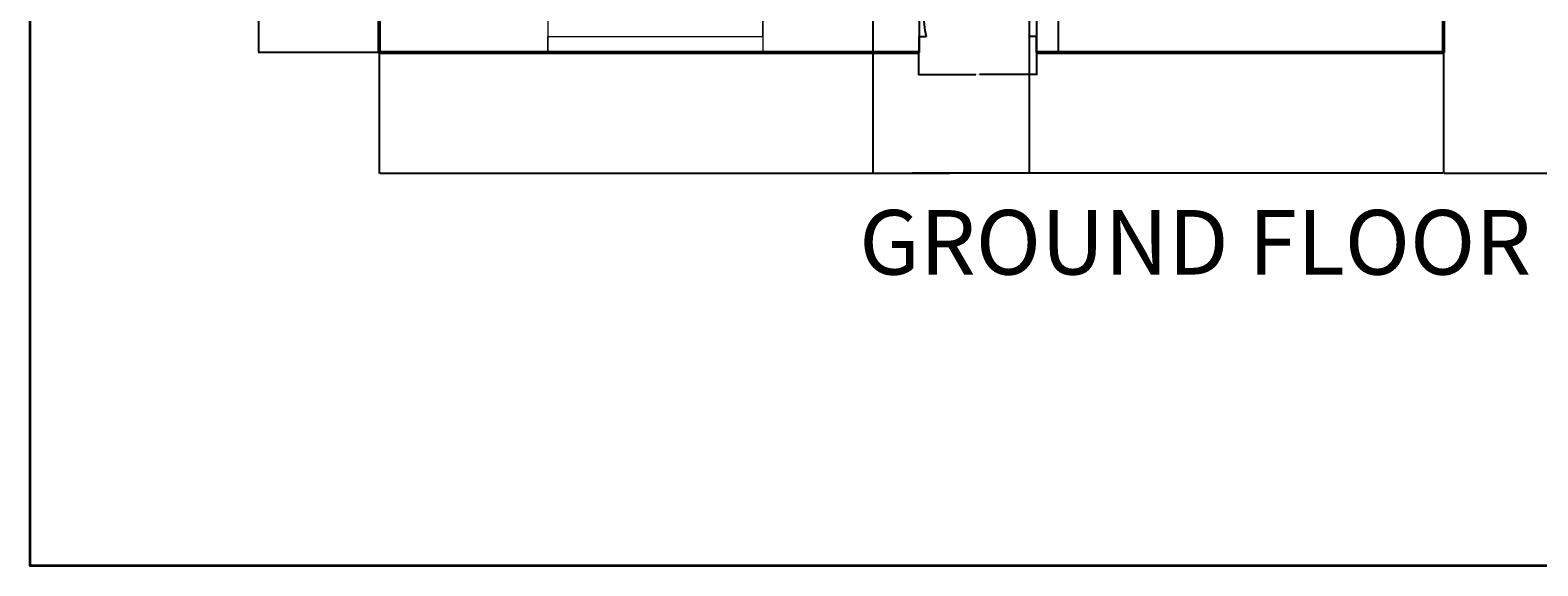
# Model space of a CAD drawing. Units: inches. Extents: x 2215 to 3724, y 1009 to 2124.
# Tile 1 of 11: x 2215 to 2636, y 1009 to 1158. Entities that reach past the tile are written whole.
import ezdxf

# ---------------------------------------------------------------- set-up
doc = ezdxf.new("R2010")
doc.units = ezdxf.units.IN
for name, color, linetype, lineweight in [('A-ANNO-DIMS', 2, 'Continuous', 18), ('A-ANNO-TEXT', 7, 'Continuous', 25), ('A-ANNO-TTLB', 7, 'Continuous', 35), ('A-DOOR', 3, 'Continuous', 25), ('A-GLAZ', 4, 'Continuous', 18), ('A-WALL', 7, 'Continuous', 50)]:
    doc.layers.add(name, color=color, linetype=linetype, lineweight=lineweight)
doc.styles.get("Standard").update_dxf_attribs({"font": 'arial.ttf'})
doc.dimstyles.get("Standard").update_dxf_attribs({"dimtxt": 0.18, "dimasz": 0.18, "dimexe": 0.18, "dimexo": 0.0625, "dimgap": 0.09, "dimtad": 0, "dimtih": 1, "dimtoh": 1, "dimdec": 4, "dimzin": 0, "dimdsep": 46, "dimtxsty": 'Standard', "dimcen": 0.09, "dimadec": 0, "dimazin": 0, "dimtfac": 1, "dimtdec": 4, "dimtofl": 0, "dimtmove": 0, "dimatfit": 3, "dimfxl": 1, "dimtolj": 1, "dimtzin": 0, "dimarcsym": 0})

# ---------------------------------------------------------------- blocks, each defined once
blk = doc.blocks.new('DOOR-FRONT-SINGLE')
for p, q in [((30.79, 4.5), (30.79, 40.5)), ((0, 9), (0, 0)), ((32.79, 9), (32.79, 0)), ((0, 0), (0, 4.5)), ((0, 4.5), (2, 4.5)), ((32.79, 4.5), (30.79, 4.5)), ((32.79, 0), (32.79, 4.5))]:
    blk.add_line(p, q)
blk.add_arc((30.39, 11.3), 29.2, 89.2162, 193.4744)
blk = doc.blocks.new('WIN-60-FRONT')
for p, q in [((0, 9), (0, 9)), ((0, 9), (0, 0)), ((60, 4.5), (60, 9)), ((60, 9), (60, 0)), ((0, 0), (0, 4.5)), ((0, 4.5), (60, 4.5))]:
    blk.add_line(p, q)
blk = doc.blocks.new('*D67')
at = {"layer": 'A-ANNO-DIMS', "color": 0, "lineweight": -2, "transparency": 16777216}
for p, q in [((2496.34, 1192.62), (2502.55, 1192.62)), ((2502.37, 1192.44), (2502.37, 1172.49)), ((2502.37, 1152.18), (2502.37, 1172.13)), ((2496.34, 1152), (2502.55, 1152))]:
    blk.add_line(p, q, dxfattribs=at)
at = {"layer": 'A-ANNO-DIMS', "color": 0, "transparency": 16777216}
for points in [[(2502.34, 1192.44), (2502.4, 1192.44), (2502.37, 1192.62)], [(2502.34, 1152.18), (2502.4, 1152.18), (2502.37, 1152)]]:
    blk.add_solid(points, dxfattribs=at)
at = {"layer": 'Defpoints', "color": 0, "transparency": 16777216}
for p in [(2496.28, 1192.62), (2502.37, 1192.62), (2496.28, 1152)]:
    blk.add_point(p, dxfattribs=at)
at = {"layer": 'A-ANNO-DIMS', "color": 0, "transparency": 16777216, "insert": (2502.37, 1172.31), "char_height": 0.18, "attachment_point": 5}
blk.add_mtext('\\A1;ENTRY DOOR 41 TYP.', dxfattribs=at)
blk = doc.blocks.new('*D68')
at = {"layer": 'A-ANNO-DIMS', "color": 0, "lineweight": -2, "transparency": 16777216}
for p, q in [((2463.38, 1151.93), (2463.38, 1145.72)), ((2496.28, 1151.93), (2496.28, 1145.72)), ((2463.56, 1145.9), (2479.3, 1145.9)), ((2496.1, 1145.9), (2480.36, 1145.9))]:
    blk.add_line(p, q, dxfattribs=at)
at = {"layer": 'A-ANNO-DIMS', "color": 0, "transparency": 16777216}
for points in [[(2463.56, 1145.93), (2463.56, 1145.87), (2463.38, 1145.9)], [(2496.1, 1145.93), (2496.1, 1145.87), (2496.28, 1145.9)]]:
    blk.add_solid(points, dxfattribs=at)
at = {"layer": 'Defpoints', "color": 0, "transparency": 16777216}
for p in [(2463.38, 1152), (2496.28, 1152), (2496.28, 1145.9)]:
    blk.add_point(p, dxfattribs=at)
at = {"layer": 'A-ANNO-DIMS', "color": 0, "transparency": 16777216, "insert": (2479.83, 1145.9), "char_height": 0.18, "attachment_point": 5}
blk.add_mtext('\\A1;33 TYP.', dxfattribs=at)
blk = doc.blocks.new('*D88')
at = {"layer": 'A-ANNO-DIMS', "color": 0, "lineweight": -2, "transparency": 16777216}
for p, q in [((2312.78, 1747.5), (2279.06, 1747.5)), ((2279.24, 1747.32), (2279.24, 1449.93)), ((2279.24, 1152.18), (2279.24, 1449.57)), ((2312.78, 1152), (2279.06, 1152))]:
    blk.add_line(p, q, dxfattribs=at)
at = {"layer": 'A-ANNO-DIMS', "color": 0, "transparency": 16777216}
for points in [[(2279.21, 1747.32), (2279.27, 1747.32), (2279.24, 1747.5)], [(2279.21, 1152.18), (2279.27, 1152.18), (2279.24, 1152)]]:
    blk.add_solid(points, dxfattribs=at)
at = {"layer": 'Defpoints', "color": 0, "transparency": 16777216}
for p in [(2279.24, 1747.5), (2312.84, 1747.5), (2312.84, 1152)]:
    blk.add_point(p, dxfattribs=at)
at = {"layer": 'A-ANNO-DIMS', "color": 0, "transparency": 16777216, "insert": (2279.24, 1449.75), "char_height": 0.18, "attachment_point": 5}
blk.add_mtext('\\A1;595.5', dxfattribs=at)
blk = doc.blocks.new('*D98')
at = {"layer": 'A-ANNO-DIMS', "color": 0, "lineweight": -2, "transparency": 16777216}
for p, q in [((2312.84, 1151.93), (2312.84, 1118.22)), ((2609.84, 1151.93), (2609.84, 1118.22)), ((2313.02, 1118.4), (2461.05, 1118.4)), ((2609.66, 1118.4), (2461.63, 1118.4))]:
    blk.add_line(p, q, dxfattribs=at)
at = {"layer": 'A-ANNO-DIMS', "color": 0, "transparency": 16777216}
for points in [[(2313.02, 1118.43), (2313.02, 1118.37), (2312.84, 1118.4)], [(2609.66, 1118.43), (2609.66, 1118.37), (2609.84, 1118.4)]]:
    blk.add_solid(points, dxfattribs=at)
at = {"layer": 'Defpoints', "color": 0, "transparency": 16777216}
for p in [(2312.84, 1152), (2609.84, 1152), (2609.84, 1118.4)]:
    blk.add_point(p, dxfattribs=at)
at = {"layer": 'A-ANNO-DIMS', "color": 0, "transparency": 16777216, "insert": (2461.34, 1118.4), "char_height": 0.18, "attachment_point": 5}
blk.add_mtext('\\A1;297', dxfattribs=at)
blk = doc.blocks.new('*D99')
at = {"layer": 'A-ANNO-DIMS', "color": 0, "lineweight": -2, "transparency": 16777216}
for p, q in [((2684.84, 1343.93), (2684.84, 1118.22)), ((2609.84, 1151.93), (2609.84, 1118.22)), ((2610.02, 1118.4), (2647.12, 1118.4)), ((2684.66, 1118.4), (2647.56, 1118.4))]:
    blk.add_line(p, q, dxfattribs=at)
at = {"layer": 'A-ANNO-DIMS', "color": 0, "transparency": 16777216}
for points in [[(2610.02, 1118.43), (2610.02, 1118.37), (2609.84, 1118.4)], [(2684.66, 1118.43), (2684.66, 1118.37), (2684.84, 1118.4)]]:
    blk.add_solid(points, dxfattribs=at)
at = {"layer": 'Defpoints', "color": 0, "transparency": 16777216}
for p in [(2684.84, 1344), (2609.84, 1152), (2684.84, 1118.4)]:
    blk.add_point(p, dxfattribs=at)
at = {"layer": 'A-ANNO-DIMS', "color": 0, "transparency": 16777216, "insert": (2647.34, 1118.4), "char_height": 0.18, "attachment_point": 5}
blk.add_mtext('\\A1;75', dxfattribs=at)
blk = doc.blocks.new('*D102')
at = {"layer": 'A-ANNO-DIMS', "color": 0, "lineweight": -2, "transparency": 16777216}
for p, q in [((2450.62, 1365.21), (2450.62, 1118.22)), ((2494.2, 1365.21), (2494.2, 1118.22)), ((2450.8, 1118.4), (2472.01, 1118.4)), ((2494.02, 1118.4), (2472.8, 1118.4))]:
    blk.add_line(p, q, dxfattribs=at)
at = {"layer": 'A-ANNO-DIMS', "color": 0, "transparency": 16777216}
for points in [[(2450.8, 1118.43), (2450.8, 1118.37), (2450.62, 1118.4)], [(2494.02, 1118.43), (2494.02, 1118.37), (2494.2, 1118.4)]]:
    blk.add_solid(points, dxfattribs=at)
at = {"layer": 'Defpoints', "color": 0, "transparency": 16777216}
for p in [(2450.62, 1365.28), (2494.2, 1365.28), (2494.2, 1118.4)]:
    blk.add_point(p, dxfattribs=at)
at = {"layer": 'A-ANNO-DIMS', "color": 0, "transparency": 16777216, "insert": (2472.41, 1118.4), "char_height": 0.18, "attachment_point": 5}
blk.add_mtext('\\A1;43.58', dxfattribs=at)

msp = doc.modelspace()

# ---------------------------------------------------------------- linework, layer by layer
at = {"layer": 'A-ANNO-TTLB'}
msp.add_lwpolyline([(2215.4438, 2124.2681), (3723.6589, 2124.2681), (3723.6589, 1008.7935), (2215.4438, 1008.7935)], close=True, dxfattribs=at)
at = {"layer": 'A-WALL'}
for p, q in [((2312.841, 1517.9969), (2312.841, 1151.9969)), ((2609.841, 1160.9969), (2609.841, 1151.9969)), ((2312.841, 1151.9969), (2463.4826, 1151.9969)), ((2463.4826, 1151.9969), (2321.841, 1151.9969)), ((2510.841, 1151.9969), (2496.2773, 1151.9969)), ((2496.2773, 1151.9969), (2501.841, 1151.9969)), ((2510.841, 1151.9969), (2600.841, 1151.9969)), ((2609.841, 1151.9969), (2600.841, 1151.9969)), ((2600.841, 1151.9969), (2609.841, 1151.9969))]:
    msp.add_line(p, q, dxfattribs=at)

# ---------------------------------------------------------------- block references
at = {"layer": 'A-DOOR'}
msp.add_blockref('DOOR-FRONT-SINGLE', (2463.483, 1151.997), dxfattribs=at)
at = {"layer": 'A-GLAZ'}
msp.add_blockref('WIN-60-FRONT', (2359.903, 1151.997), dxfattribs=at)

# ---------------------------------------------------------------- texts
at = {"layer": 'A-ANNO-TEXT', "insert": (2446.809, 1108.0653), "char_height": 18, "attachment_point": 1}
msp.add_mtext_dynamic_manual_height_columns('GROUND FLOOR PLAN', width=436.700422, gutter_width=12.5, heights=[0], dxfattribs=at)

# ---------------------------------------------------------------- dimensions: what is measured, and where the dimension line sits
at = {"layer": 'A-ANNO-DIMS'}
dim = msp.add_linear_dim(base=(2279.241, 1747.4969), p1=(2312.841, 1151.9969), p2=(2312.841, 1747.4969), angle=90, dimstyle='Standard', override={"dimdec": 1, "dimlfac": 1, "dimrnd": 0, "dimzin": 0, "dimdsep": 46, "dimlunit": 2}, dxfattribs=at)
dim.commit()
dim.dimension.update_dxf_attribs({"geometry": '*D88', "text_midpoint": (2279.241, 1449.7469)})
for base, p1, p2, override, picture, middle in [((2494.1952, 1118.3969), (2450.6169, 1365.276), (2494.1952, 1365.276), {"dimdec": 2, "dimlfac": 1, "dimrnd": 0, "dimzin": 0, "dimdsep": 46, "dimlunit": 2}, '*D102', (2472.406, 1118.3969)), ((2684.841, 1118.3969), (2609.841, 1151.9969), (2684.841, 1343.9969), {"dimdec": 0, "dimlfac": 1, "dimrnd": 0, "dimzin": 0, "dimdsep": 46, "dimlunit": 2}, '*D99', (2647.341, 1118.3969)), ((2609.841, 1118.3969), (2312.841, 1151.9969), (2609.841, 1151.9969), {"dimdec": 0, "dimlfac": 1, "dimrnd": 0, "dimzin": 0, "dimdsep": 46, "dimlunit": 2}, '*D98', (2461.341, 1118.3969))]:
    dim = msp.add_linear_dim(base=base, p1=p1, p2=p2, dimstyle='Standard', override=override, dxfattribs=at)
    dim.commit()
    dim.dimension.update_dxf_attribs({"geometry": picture, "text_midpoint": middle})
dim = msp.add_linear_dim(base=(2502.3708, 1192.6202), p1=(2496.2773, 1151.9969), p2=(2496.2773, 1192.6202), angle=90, text='ENTRY DOOR <> TYP.', dimstyle='Standard', override={"dimdec": 0, "dimlfac": 1, "dimrnd": 0, "dimzin": 0, "dimdsep": 46, "dimlunit": 2}, dxfattribs=at)
dim.commit()
dim.dimension.update_dxf_attribs({"geometry": '*D67', "text_midpoint": (2502.3708, 1172.3086)})
dim = msp.add_linear_dim(base=(2496.2773, 1145.9034), p1=(2463.3829, 1151.9969), p2=(2496.2773, 1151.9969), text='<> TYP.', dimstyle='Standard', override={"dimdec": 0, "dimlfac": 1, "dimrnd": 0, "dimzin": 0, "dimdsep": 46, "dimlunit": 2}, dxfattribs=at)
dim.commit()
dim.dimension.update_dxf_attribs({"geometry": '*D68', "text_midpoint": (2479.8301, 1145.9034)})

doc.saveas('drawing.dxf')
